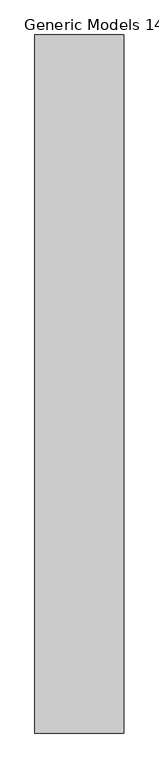
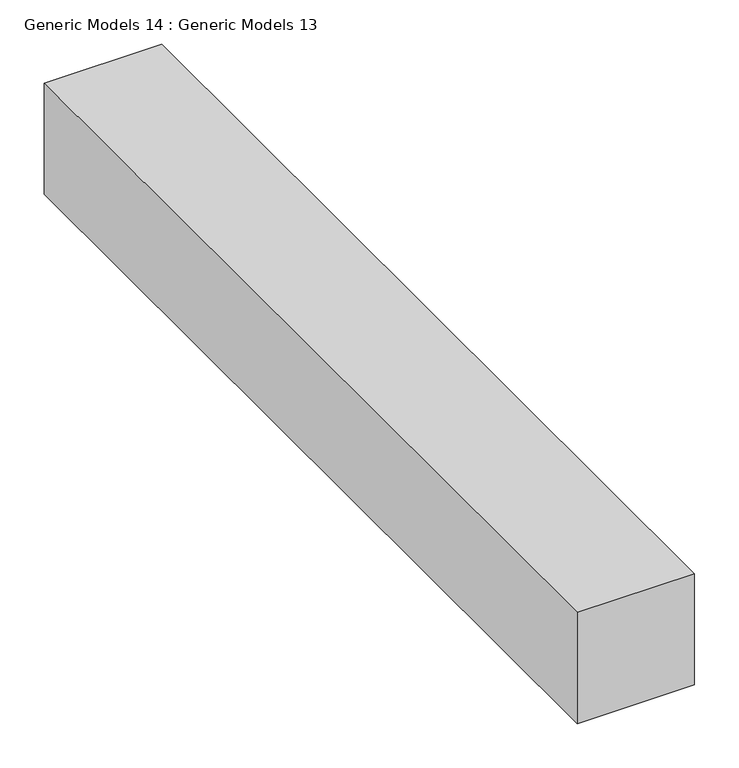
"""IFC4 building model written with IfcOpenShell, lengths in millimetres: proxy geometry, Generic Models 14 : Generic Models 13."""

from ifc_helpers import new_model, si_unit, frame, origin, place, context, project, spatial, polyline, outline, extrude, source, transform, mapped, element, save


def generic_models_14_generic_models_13_4ffb657b(model_context):
    return source(origin(), model_context, "Body", "SweptSolid", [
        extrude(outline(polyline([(2047.0218735, -1113.3417935), (2047.0218735, -2310.4441671), (1894.6218735, -2310.4441671), (1894.6218735, -1113.3417935), (2047.0218735, -1113.3417935)])), frame((0.0, 0.0, 9144.0), z_axis=(0.0, 0.0, 1.0), x_axis=(1.0, 0.0, 0.0)), (0.0, 0.0, 1.0), 152.4),
    ])


if __name__ == "__main__":
    model = new_model("IFC4")
    model_context = context("Model", 3, world=origin())
    ifc_project = project(units=[si_unit("LENGTHUNIT", "METRE", prefix="MILLI")], contexts=[model_context])
    site = spatial("IfcSite", under=ifc_project)
    building = spatial("IfcBuilding", under=site)
    placement = place(None, origin())
    generic_models_14_generic_models_13_shape = generic_models_14_generic_models_13_4ffb657b(model_context)
    element("IfcBuildingElementProxy", 1, Name="Generic Models 14 : Generic Models 13", ObjectType="Generic Models 14 : Generic Models 13", at=placement, inside=building, context=model_context, shape_type="MappedRepresentation", body=[
        mapped(generic_models_14_generic_models_13_shape, transform((0.0, 0.0, 0.0), x_axis=(1.0, 0.0, 0.0), y_axis=(0.0, 1.0, 0.0), z_axis=(0.0, 0.0, 1.0))),
    ])
    save(model, "model.ifc")
